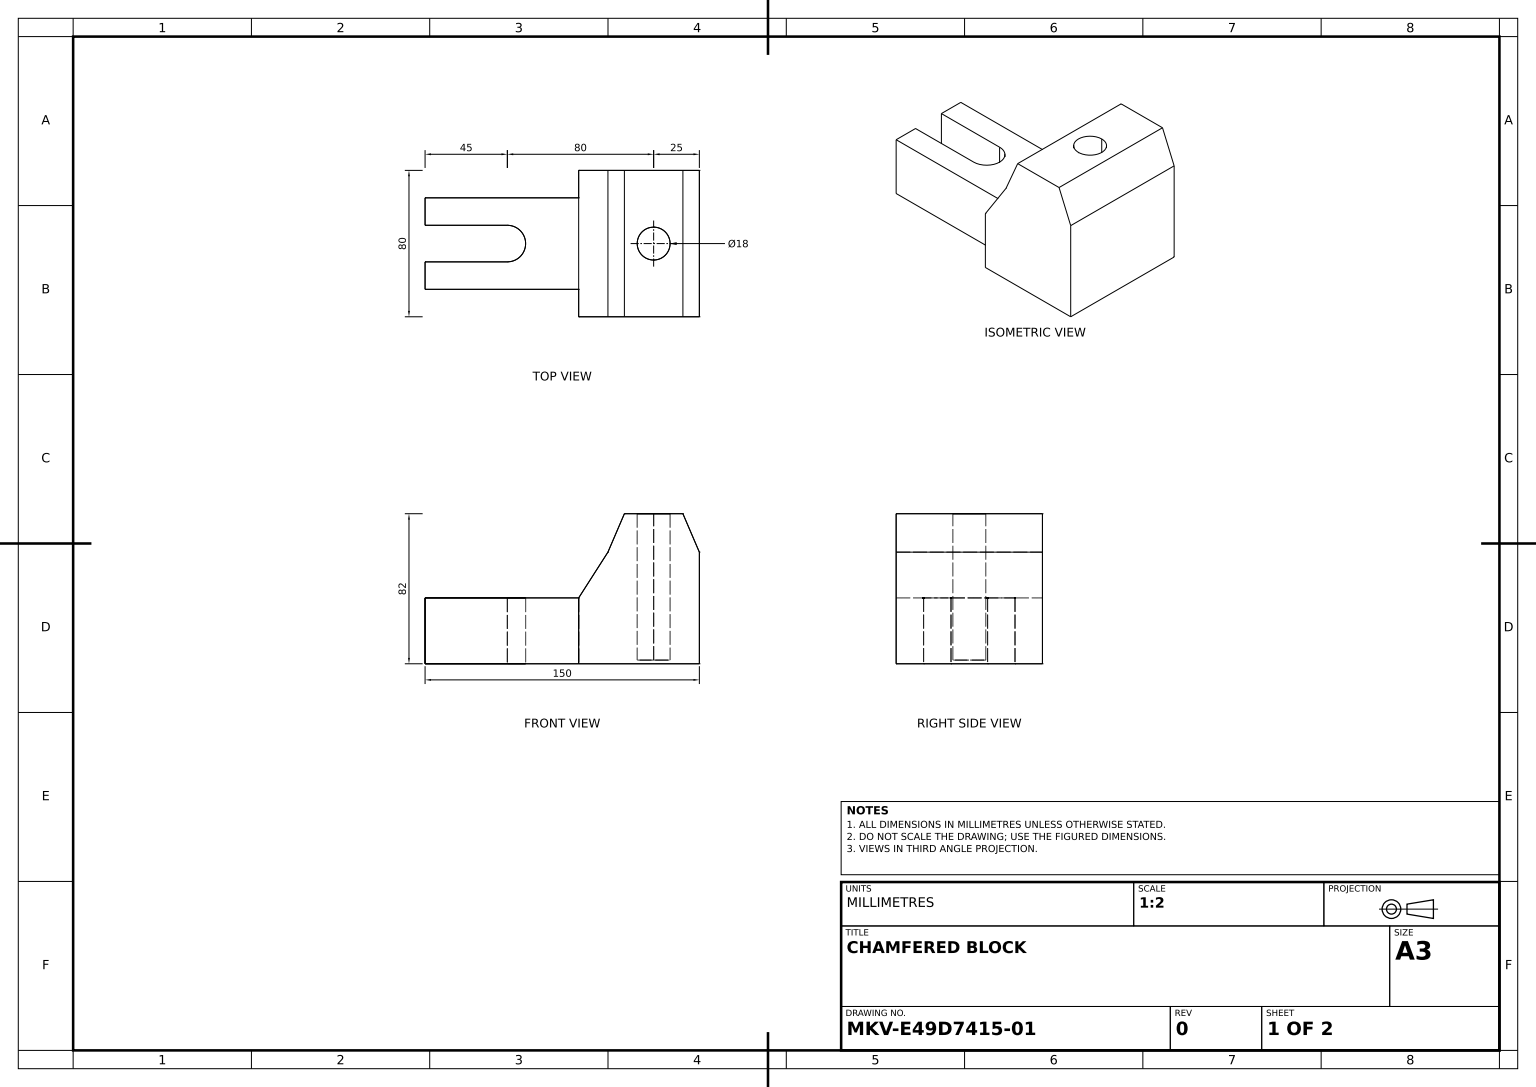
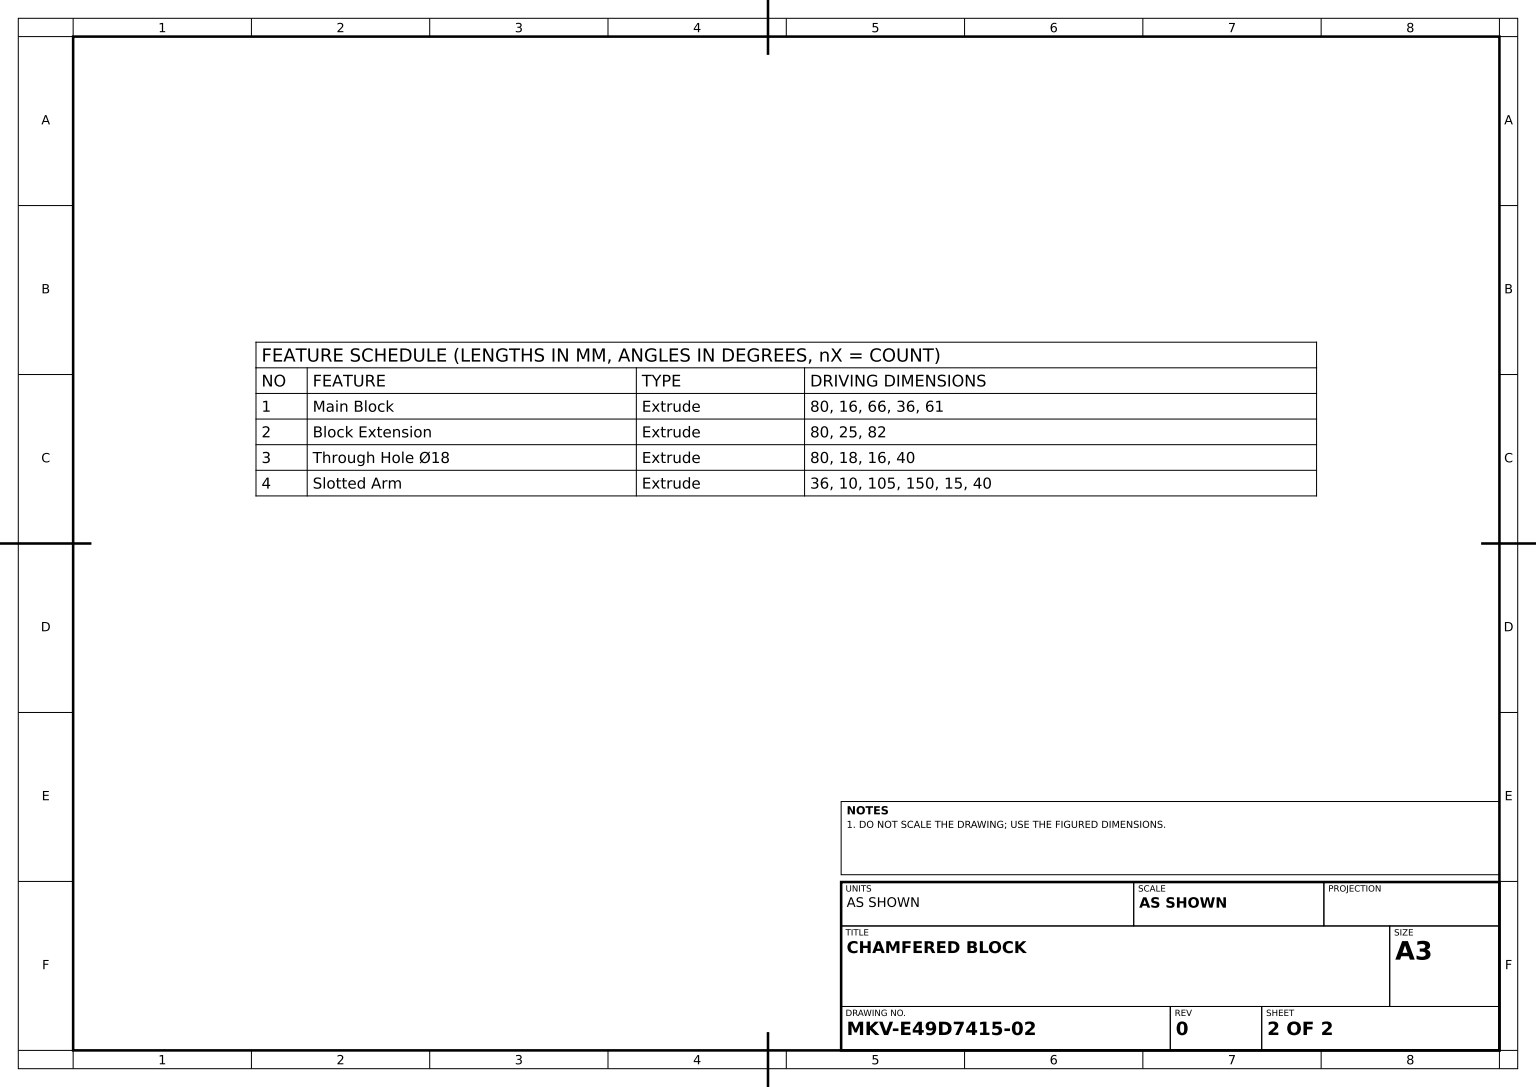
SolidWorks part; units mm, degrees
material "Plain Carbon Steel"
ref_plane "Front Plane" through (0, 0, 0) normal (0, 0, 1) x (1, 0, 0)
ref_plane "Top Plane" through (0, 0, 0) normal (0, 1, 0) x (1, 0, 0)
ref_plane "Right Plane" through (0, 0, 0) normal (1, 0, 0) x (0, 0, -1)
sketch "Main Block Profile" plane through (0, 0, 0) normal (0, 0, 1) x (1, 0, 0)
  line L0 (0, 0) -> (66, 0)
  line L1 (66, 0) -> (66, 61)
  line L2 (0, 0) -> (0, 36)
  line L9 (66, 61) -> (16, 61)
  line L10 (16, 61) -> (0, 36)
  dimension "D1" = 16
  dimension "D2" = 66
  dimension "D3" = 36
  dimension "D4" = 61
extrude "Main Block" add sketch "Main Block Profile" along normal blind 80
sketch "Block Extension Profile" plane through (0, 0, 80) normal (0, 0, 1) x (1, 0, 0)
  line L0 (0, 36) -> (0, 0) construction
  line L1 (0, 0) -> (66, 0) construction
  line L2 (41, 82) -> (57, 82)
  line L3 (57, 82) -> (66, 61)
  line L4 (66, 61) -> (16, 61)
  line L5 (41, 82) -> (25, 82)
  line L6 (25, 82) -> (16, 61)
  dimension "D1" = 25
  dimension "D2" = 82
extrude "Block Extension" add sketch "Block Extension Profile" against normal blind 80
sketch "Hole Ø18 Sketch" plane through (0, 82, 0) normal (0, 1, 0) x (1, 0, 0)
  line L0 (57, 0) -> (57, -80) construction
  line L1 (57, -80) -> (25, -80) construction
  circle A0 centre (41, -40) radius 9
  dimension "D1" = 18
  dimension "D2" = 18
  dimension "D3" = 16
  dimension "D4" = 40
extrude "Through Hole Ø18" cut sketch "Hole Ø18 Sketch" against normal blind 80
sketch "Slotted Arm Profile" plane through (0, 0, 0) normal (0, -1, 0) x (1, 0, 0)
  line L0 (0, 65) -> (0, 15)
  line L1 (0, 80) -> (0, 0) construction
  line L2 (0, 65) -> (-84, 65)
  line L3 (66, 80) -> (66, 0) construction
  line L4 (0, 0) -> (66, 0) construction
  line L5 (-39, 30) -> (-84, 30)
  line L6 (-39, 50) -> (-84, 50)
  line L8 (0, 15) -> (-84, 15)
  line L9 (-84, 15) -> (-84, 30)
  line L10 (-84, 65) -> (-84, 50)
  arc A0 (-39, 30) -> (-39, 50) centre (-39, 40) ccw
  dimension "D1" = 20
  dimension "D2" = 10
  dimension "D3" = 105
  dimension "D4" = 150
  dimension "D5" = 15
  dimension "D6" = 40
extrude "Slotted Arm" add sketch "Slotted Arm Profile" against normal blind 36
